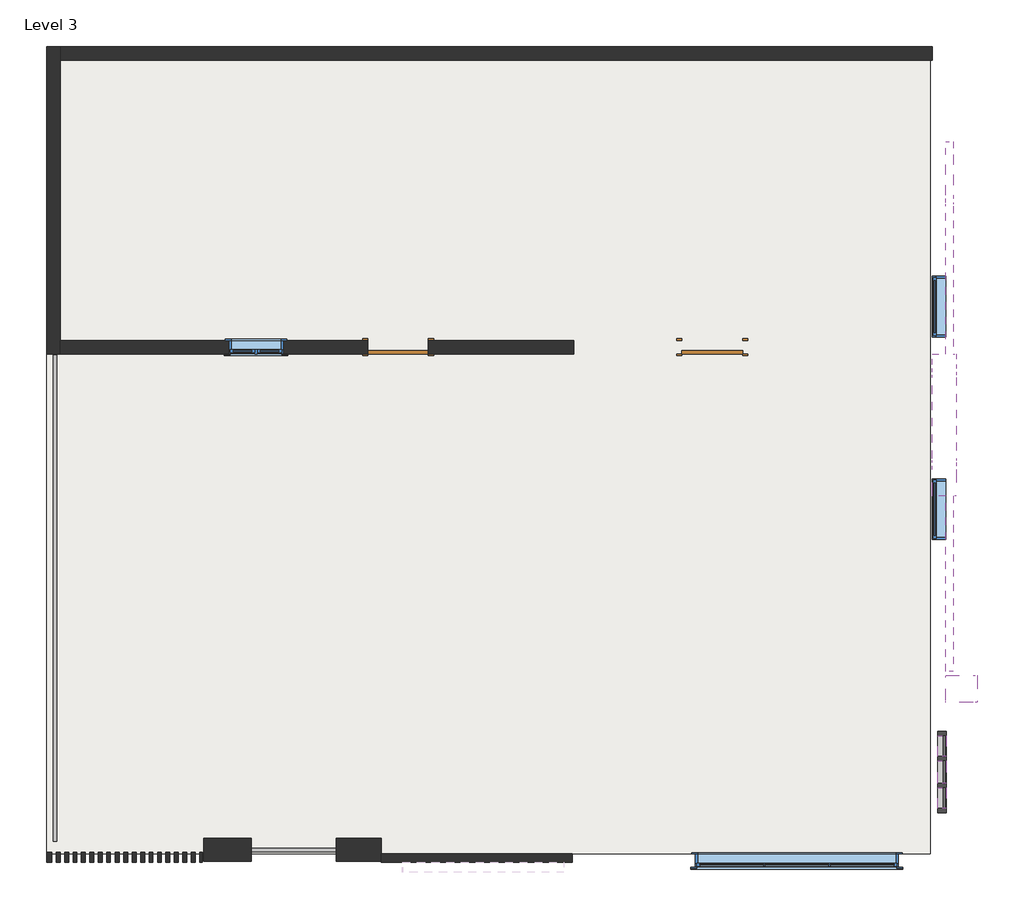
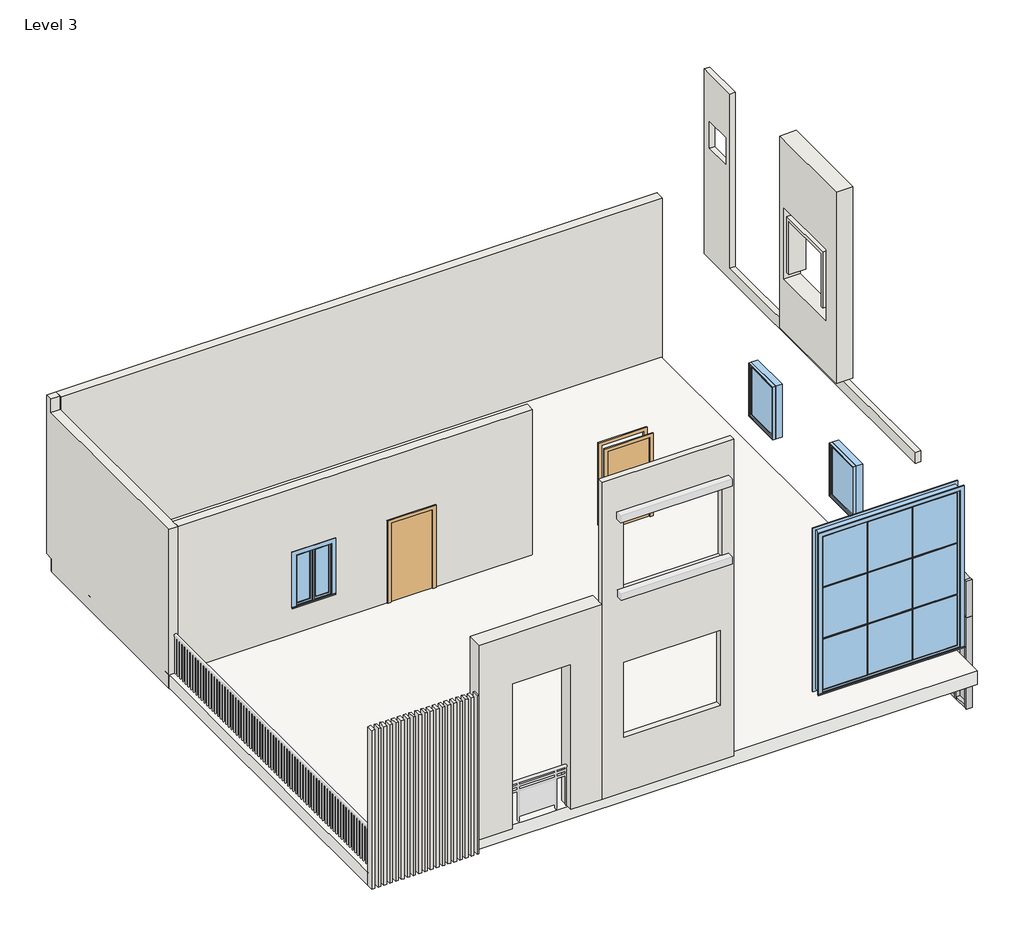
# One storey, part 1 of 2: 24 members, 9 plates, 7 walls, 5 windows, 2 doors, 1 roof.
"""IFC4 building model written with IfcOpenShell, lengths in millimetres."""

from ifc_helpers import new_model, si_unit, frame, origin, place, context, project, spatial, polyline, outline, extrude, faceted_brep, transform, mapped, element, save
from components import door_54dd4da4, member_ff1b7d8f, member_5ad95953, member_62b9d9f2, member_5aeb4b7d, member_9850ab14, member_238a442c, member_fec1d5e2, member_24c95a33, member_92f44db0, member_86adc6a2, system_panel_glazed_2f2cf5d5, system_panel_glazed_6255ac7b, system_panel_glazed_0848ed2a, system_panel_glazed_7089d882, system_panel_glazed_51dabc0a, system_panel_glazed_dcf6fd09, walls_4_walls_4_cd32183e, walls_6_walls_6_5288b44a, window_cae7f124, window_bb17773d, window_8bd8a12f, window_e2841890

model = new_model("IFC4")

# Units and contexts
model_context = context("Model", 3, world=origin())
ifc_project = project(units=[si_unit("LENGTHUNIT", "METRE", prefix="MILLI")], contexts=[model_context])

# Site, building, storey
site = spatial("IfcSite", under=ifc_project)
building = spatial("IfcBuilding", under=site)
storey = spatial("IfcBuildingStorey", under=building, Name="Level 3", Elevation=7315.2)

# Doors
placement = place(None, origin())
door_shape = door_54dd4da4(model_context)
element("IfcDoor", 1, ObjectType="Single-Flush : 36\" x 84\"", at=placement, inside=storey, context=model_context, shape_type="MappedRepresentation", body=[
    mapped(door_shape, transform((-6567.2745124, 6836.8609482, 7315.2), x_axis=(-1.0, 0.0, 0.0), y_axis=(0.0, -1.0, 0.0), z_axis=(0.0, 0.0, 1.0))),
])
element("IfcDoor", 2, ObjectType="Single-Flush : 36\" x 84\"", at=placement, inside=storey, context=model_context, shape_type="MappedRepresentation", body=[
    mapped(door_shape, transform((-1842.8745124, 6836.8609482, 7315.2), x_axis=(-1.0, 0.0, 0.0), y_axis=(0.0, -1.0, 0.0), z_axis=(0.0, 0.0, 1.0))),
])

# Members
member_shape = member_ff1b7d8f(model_context)
element("IfcMember", 3, ObjectType="Rectangular Mullion : 2.5\" x 5\" rectangular", at=placement, inside=storey, context=model_context, shape_type="MappedRepresentation", body=[
    mapped(member_shape, transform((1611.5254876, 617.0832725, 6324.9019988), x_axis=(0.0, 0.0, -1.0), y_axis=(-1.0, 0.0, 0.0), z_axis=(0.0, 1.0, 0.0))),
])
member_2_shape = member_5ad95953(model_context)
element("IfcMember", 4, ObjectType="Rectangular Mullion : 2.5\" x 5\" rectangular", at=placement, inside=storey, context=model_context, shape_type="MappedRepresentation", body=[
    mapped(member_2_shape, transform((1611.5254876, 210.6832725, 6324.9019988), x_axis=(0.0, 0.0, -1.0), y_axis=(-1.0, 0.0, 0.0), z_axis=(0.0, 1.0, 0.0))),
])
element("IfcMember", 5, ObjectType="Rectangular Mullion : 2.5\" x 5\" rectangular", at=placement, inside=storey, context=model_context, shape_type="MappedRepresentation", body=[
    mapped(member_2_shape, transform((1611.5254876, 991.7332725, 6324.9019988), x_axis=(0.0, 0.0, -1.0), y_axis=(-1.0, 0.0, 0.0), z_axis=(0.0, 1.0, 0.0))),
])
member_3_shape = member_62b9d9f2(model_context)
element("IfcMember", 6, ObjectType="Rectangular Mullion : 2.5\" x 5\" rectangular", at=placement, inside=storey, context=model_context, shape_type="MappedRepresentation", body=[
    mapped(member_3_shape, transform((1611.5254876, 242.4332725, 6324.9019988), x_axis=(0.0, -1.0, 0.0), y_axis=(-1.0, 0.0, 0.0), z_axis=(0.0, 0.0, -1.0))),
])
element("IfcMember", 7, ObjectType="Rectangular Mullion : 2.5\" x 5\" rectangular", at=placement, inside=storey, context=model_context, shape_type="MappedRepresentation", body=[
    mapped(member_3_shape, transform((1611.5254876, 648.8332725, 6324.9019988), x_axis=(0.0, -1.0, 0.0), y_axis=(-1.0, 0.0, 0.0), z_axis=(0.0, 0.0, -1.0))),
])
member_4_shape = member_5aeb4b7d(model_context)
element("IfcMember", 8, ObjectType="Rectangular Mullion : 2.5\" x 5\" rectangular", at=placement, inside=storey, context=model_context, shape_type="MappedRepresentation", body=[
    mapped(member_4_shape, transform((1611.5254876, 274.1832725, 7239.0), x_axis=(0.0, 0.0, 1.0), y_axis=(-1.0, 0.0, 0.0), z_axis=(0.0, -1.0, 0.0))),
])
element("IfcMember", 9, ObjectType="Rectangular Mullion : 2.5\" x 5\" rectangular", at=placement, inside=storey, context=model_context, shape_type="MappedRepresentation", body=[
    mapped(member_4_shape, transform((1611.5254876, 274.1832725, 8433.1019988), x_axis=(0.0, 0.0, 1.0), y_axis=(-1.0, 0.0, 0.0), z_axis=(0.0, -1.0, 0.0))),
])
member_5_shape = member_9850ab14(model_context)
element("IfcMember", 10, ObjectType="Rectangular Mullion : 2.5\" x 5\" rectangular", at=placement, inside=storey, context=model_context, shape_type="MappedRepresentation", body=[
    mapped(member_5_shape, transform((1611.5254876, -100.4667275, 7239.0), x_axis=(0.0, 0.0, 1.0), y_axis=(-1.0, 0.0, 0.0), z_axis=(0.0, -1.0, 0.0))),
])
element("IfcMember", 11, ObjectType="Rectangular Mullion : 2.5\" x 5\" rectangular", at=placement, inside=storey, context=model_context, shape_type="MappedRepresentation", body=[
    mapped(member_5_shape, transform((1611.5254876, 680.5832725, 7239.0), x_axis=(0.0, 0.0, 1.0), y_axis=(-1.0, 0.0, 0.0), z_axis=(0.0, -1.0, 0.0))),
])
element("IfcMember", 12, ObjectType="Rectangular Mullion : 2.5\" x 5\" rectangular", at=placement, inside=storey, context=model_context, shape_type="MappedRepresentation", body=[
    mapped(member_5_shape, transform((1611.5254876, -100.4667275, 8433.1019988), x_axis=(0.0, 0.0, 1.0), y_axis=(-1.0, 0.0, 0.0), z_axis=(0.0, -1.0, 0.0))),
])
element("IfcMember", 13, ObjectType="Rectangular Mullion : 2.5\" x 5\" rectangular", at=placement, inside=storey, context=model_context, shape_type="MappedRepresentation", body=[
    mapped(member_5_shape, transform((1611.5254876, 680.5832725, 8433.1019988), x_axis=(0.0, 0.0, 1.0), y_axis=(-1.0, 0.0, 0.0), z_axis=(0.0, -1.0, 0.0))),
])
member_6_shape = member_238a442c(model_context)
element("IfcMember", 14, ObjectType="Rectangular Mullion : 2.5\" x 5\" rectangular", at=placement, inside=storey, context=model_context, shape_type="MappedRepresentation", body=[
    mapped(member_6_shape, transform((1611.5254876, 1055.2332725, 7239.0), x_axis=(0.0, 1.0, 0.0), y_axis=(-1.0, 0.0, 0.0), z_axis=(0.0, 0.0, 1.0))),
])
element("IfcMember", 15, ObjectType="Rectangular Mullion : 2.5\" x 5\" rectangular", at=placement, inside=storey, context=model_context, shape_type="MappedRepresentation", body=[
    mapped(member_6_shape, transform((1611.5254876, -163.9667275, 6324.9019988), x_axis=(0.0, -1.0, 0.0), y_axis=(-1.0, 0.0, 0.0), z_axis=(0.0, 0.0, -1.0))),
])
member_7_shape = member_fec1d5e2(model_context)
element("IfcMember", 16, ObjectType="Rectangular Mullion : 2.5\" x 5\" rectangular", at=placement, inside=storey, context=model_context, shape_type="MappedRepresentation", body=[
    mapped(member_7_shape, transform((1611.5254876, 242.4332725, 7239.0), x_axis=(0.0, -1.0, 0.0), y_axis=(-1.0, 0.0, 0.0), z_axis=(0.0, 0.0, -1.0))),
])
element("IfcMember", 17, ObjectType="Rectangular Mullion : 2.5\" x 5\" rectangular", at=placement, inside=storey, context=model_context, shape_type="MappedRepresentation", body=[
    mapped(member_7_shape, transform((1611.5254876, 648.8332725, 7239.0), x_axis=(0.0, -1.0, 0.0), y_axis=(-1.0, 0.0, 0.0), z_axis=(0.0, 0.0, -1.0))),
])
member_8_shape = member_24c95a33(model_context)
element("IfcMember", 18, ObjectType="Rectangular Mullion : 2.5\" x 5\" rectangular", at=placement, inside=storey, context=model_context, shape_type="MappedRepresentation", body=[
    mapped(member_8_shape, transform((1611.5254876, 1055.2332725, 8433.1019988), x_axis=(0.0, 1.0, 0.0), y_axis=(-1.0, 0.0, 0.0), z_axis=(0.0, 0.0, 1.0))),
])
element("IfcMember", 19, ObjectType="Rectangular Mullion : 2.5\" x 5\" rectangular", at=placement, inside=storey, context=model_context, shape_type="MappedRepresentation", body=[
    mapped(member_8_shape, transform((1611.5254876, -163.9667275, 7239.0), x_axis=(0.0, -1.0, 0.0), y_axis=(-1.0, 0.0, 0.0), z_axis=(0.0, 0.0, -1.0))),
])
member_9_shape = member_92f44db0(model_context)
element("IfcMember", 20, ObjectType="Rectangular Mullion : 2.5\" x 5\" rectangular", at=placement, inside=storey, context=model_context, shape_type="MappedRepresentation", body=[
    mapped(member_9_shape, transform((1611.5254876, 242.4332725, 8433.1019988), x_axis=(0.0, -1.0, 0.0), y_axis=(-1.0, 0.0, 0.0), z_axis=(0.0, 0.0, -1.0))),
])
element("IfcMember", 21, ObjectType="Rectangular Mullion : 2.5\" x 5\" rectangular", at=placement, inside=storey, context=model_context, shape_type="MappedRepresentation", body=[
    mapped(member_9_shape, transform((1611.5254876, 648.8332725, 8433.1019988), x_axis=(0.0, -1.0, 0.0), y_axis=(-1.0, 0.0, 0.0), z_axis=(0.0, 0.0, -1.0))),
])
element("IfcMember", 22, ObjectType="Rectangular Mullion : 2.5\" x 5\" rectangular", at=placement, inside=storey, context=model_context, shape_type="MappedRepresentation", body=[
    mapped(member_2_shape, transform((1611.5254876, 680.5832725, 9271.3019988), x_axis=(0.0, 0.0, 1.0), y_axis=(-1.0, 0.0, 0.0), z_axis=(0.0, -1.0, 0.0))),
])
element("IfcMember", 23, ObjectType="Rectangular Mullion : 2.5\" x 5\" rectangular", at=placement, inside=storey, context=model_context, shape_type="MappedRepresentation", body=[
    mapped(member_2_shape, transform((1611.5254876, -100.4667275, 9271.3019988), x_axis=(0.0, 0.0, 1.0), y_axis=(-1.0, 0.0, 0.0), z_axis=(0.0, -1.0, 0.0))),
])
element("IfcMember", 24, ObjectType="Rectangular Mullion : 2.5\" x 5\" rectangular", at=placement, inside=storey, context=model_context, shape_type="MappedRepresentation", body=[
    mapped(member_shape, transform((1611.5254876, 274.1832725, 9271.3019988), x_axis=(0.0, 0.0, 1.0), y_axis=(-1.0, 0.0, 0.0), z_axis=(0.0, -1.0, 0.0))),
])
member_10_shape = member_86adc6a2(model_context)
element("IfcMember", 25, ObjectType="Rectangular Mullion : 2.5\" x 5\" rectangular", at=placement, inside=storey, context=model_context, shape_type="MappedRepresentation", body=[
    mapped(member_10_shape, transform((1611.5254876, 1055.2332725, 9271.3019988), x_axis=(0.0, 1.0, 0.0), y_axis=(-1.0, 0.0, 0.0), z_axis=(0.0, 0.0, 1.0))),
])
element("IfcMember", 26, ObjectType="Rectangular Mullion : 2.5\" x 5\" rectangular", at=placement, inside=storey, context=model_context, shape_type="MappedRepresentation", body=[
    mapped(member_10_shape, transform((1611.5254876, -163.9667275, 8433.1019988), x_axis=(0.0, -1.0, 0.0), y_axis=(-1.0, 0.0, 0.0), z_axis=(0.0, 0.0, -1.0))),
])

# Plates
system_panel_glazed_shape = system_panel_glazed_2f2cf5d5(model_context)
element("IfcPlate", 27, ObjectType="System Panel : Glazed", at=placement, inside=storey, context=model_context, shape_type="MappedRepresentation", body=[
    mapped(system_panel_glazed_shape, transform((1611.5254876, 836.1582725, 6388.4019988), x_axis=(0.0, -1.0, 0.0), y_axis=(1.0, 0.0, 0.0), z_axis=(0.0, 0.0, 1.0))),
])
element("IfcPlate", 28, ObjectType="System Panel : Glazed", at=placement, inside=storey, context=model_context, shape_type="MappedRepresentation", body=[
    mapped(system_panel_glazed_shape, transform((1611.5254876, 55.1082725, 6388.4019988), x_axis=(0.0, -1.0, 0.0), y_axis=(1.0, 0.0, 0.0), z_axis=(0.0, 0.0, 1.0))),
])
system_panel_glazed_2_shape = system_panel_glazed_6255ac7b(model_context)
element("IfcPlate", 29, ObjectType="System Panel : Glazed", at=placement, inside=storey, context=model_context, shape_type="MappedRepresentation", body=[
    mapped(system_panel_glazed_2_shape, transform((1611.5254876, 445.6332725, 6388.4019988), x_axis=(0.0, -1.0, 0.0), y_axis=(1.0, 0.0, 0.0), z_axis=(0.0, 0.0, 1.0))),
])
system_panel_glazed_3_shape = system_panel_glazed_0848ed2a(model_context)
element("IfcPlate", 30, ObjectType="System Panel : Glazed", at=placement, inside=storey, context=model_context, shape_type="MappedRepresentation", body=[
    mapped(system_panel_glazed_3_shape, transform((1611.5254876, 836.1582725, 7270.75), x_axis=(0.0, -1.0, 0.0), y_axis=(1.0, 0.0, 0.0), z_axis=(0.0, 0.0, 1.0))),
])
element("IfcPlate", 31, ObjectType="System Panel : Glazed", at=placement, inside=storey, context=model_context, shape_type="MappedRepresentation", body=[
    mapped(system_panel_glazed_3_shape, transform((1611.5254876, 55.1082725, 7270.75), x_axis=(0.0, -1.0, 0.0), y_axis=(1.0, 0.0, 0.0), z_axis=(0.0, 0.0, 1.0))),
])
system_panel_glazed_4_shape = system_panel_glazed_7089d882(model_context)
element("IfcPlate", 32, ObjectType="System Panel : Glazed", at=placement, inside=storey, context=model_context, shape_type="MappedRepresentation", body=[
    mapped(system_panel_glazed_4_shape, transform((1611.5254876, 445.6332725, 7270.75), x_axis=(0.0, -1.0, 0.0), y_axis=(1.0, 0.0, 0.0), z_axis=(0.0, 0.0, 1.0))),
])
system_panel_glazed_5_shape = system_panel_glazed_51dabc0a(model_context)
element("IfcPlate", 33, ObjectType="System Panel : Glazed", at=placement, inside=storey, context=model_context, shape_type="MappedRepresentation", body=[
    mapped(system_panel_glazed_5_shape, transform((1611.5254876, 836.1582725, 8464.8519988), x_axis=(0.0, -1.0, 0.0), y_axis=(1.0, 0.0, 0.0), z_axis=(0.0, 0.0, 1.0))),
])
element("IfcPlate", 34, ObjectType="System Panel : Glazed", at=placement, inside=storey, context=model_context, shape_type="MappedRepresentation", body=[
    mapped(system_panel_glazed_5_shape, transform((1611.5254876, 55.1082725, 8464.8519988), x_axis=(0.0, -1.0, 0.0), y_axis=(1.0, 0.0, 0.0), z_axis=(0.0, 0.0, 1.0))),
])
system_panel_glazed_6_shape = system_panel_glazed_dcf6fd09(model_context)
element("IfcPlate", 35, ObjectType="System Panel : Glazed", at=placement, inside=storey, context=model_context, shape_type="MappedRepresentation", body=[
    mapped(system_panel_glazed_6_shape, transform((1611.5254876, 445.6332725, 8464.8519988), x_axis=(0.0, -1.0, 0.0), y_axis=(1.0, 0.0, 0.0), z_axis=(0.0, 0.0, 1.0))),
])

# Roof
element("IfcRoof", 36, ObjectType="Generic - 12\"", at=placement, inside=storey, context=model_context, shape_type="SweptSolid", body=[
    extrude(outline(polyline([(-11847.2995124, 11192.9609482), (1433.7254876, 11192.9609482), (1433.7254876, -783.1390518), (-11847.2995124, -783.1390518), (-11847.2995124, 11192.9609482)])), frame((0.0, 0.0, 7315.2), z_axis=(0.0, 0.0, 1.0), x_axis=(1.0, 0.0, 0.0)), (0.0, 0.0, 1.0), 304.8),
])

# Walls
element("IfcWall", 37, ObjectType="Generic - 5\"", at=placement, inside=storey, context=model_context, shape_type="SweptSolid", body=[
    extrude(outline(polyline([(7623.0321664, -6816.4084212), (7623.0321664, -3950.544029), (14935.2, -3950.544029), (14935.2, -6816.4084212), (7623.0321664, -6816.4084212)]), holes=[polyline([(13989.7022407, -4213.8822527), (12313.3022407, -4213.8822527), (12313.3022407, -6354.4547188), (13989.7022407, -6354.4547188), (13989.7022407, -4213.8822527)]), polyline([(10627.4720431, -4247.1363239), (8900.2720431, -4247.1363239), (8900.2720431, -6354.4547188), (10627.4720431, -6354.4547188), (10627.4720431, -4247.1363239)])]), frame((0.0, -909.5189974, 0.0), z_axis=(0.0, 1.0, 0.0), x_axis=(0.0, 0.0, 1.0)), (0.0, 0.0, 1.0), 127.0),
])
element("IfcWall", 38, ObjectType="Generic - 6\"", at=placement, inside=storey, context=model_context, shape_type="SweptSolid", body=[
    extrude(outline(polyline([(-11774.3919854, -910.1390518), (-11847.2995124, -910.1390518), (-11847.2995124, -757.7390518), (-11774.3919854, -757.7390518), (-11774.3919854, -910.1390518)])), frame((0.0, 0.0, 7315.2), z_axis=(0.0, 0.0, 1.0), x_axis=(1.0, 0.0, 0.0)), (0.0, 0.0, 1.0), 3657.6),
    extrude(outline(polyline([(-9510.4995124, -910.1390518), (-9547.5440884, -910.1390518), (-9547.5440884, -757.7390518), (-9510.4995124, -757.7390518), (-9510.4995124, -910.1390518)])), frame((0.0, 0.0, 7315.2), z_axis=(0.0, 0.0, 1.0), x_axis=(1.0, 0.0, 0.0)), (0.0, 0.0, 1.0), 3657.6),
    extrude(outline(polyline([(-11647.2745124, -910.1390518), (-11706.5440884, -910.1390518), (-11706.5440884, -757.7390518), (-11647.2745124, -757.7390518), (-11647.2745124, -910.1390518)])), frame((0.0, 0.0, 7315.2), z_axis=(0.0, 0.0, 1.0), x_axis=(1.0, 0.0, 0.0)), (0.0, 0.0, 1.0), 3657.6),
    extrude(outline(polyline([(-11520.3919854, -910.1390518), (-11579.4266155, -910.1390518), (-11579.4266155, -757.7390518), (-11520.3919854, -757.7390518), (-11520.3919854, -910.1390518)])), frame((0.0, 0.0, 7315.2), z_axis=(0.0, 0.0, 1.0), x_axis=(1.0, 0.0, 0.0)), (0.0, 0.0, 1.0), 3657.6),
    extrude(outline(polyline([(-11393.3919854, -910.1390518), (-11452.5440884, -910.1390518), (-11452.5440884, -757.7390518), (-11393.3919854, -757.7390518), (-11393.3919854, -910.1390518)])), frame((0.0, 0.0, 7315.2), z_axis=(0.0, 0.0, 1.0), x_axis=(1.0, 0.0, 0.0)), (0.0, 0.0, 1.0), 3657.6),
    extrude(outline(polyline([(-11266.3919854, -910.1390518), (-11325.5440884, -910.1390518), (-11325.5440884, -757.7390518), (-11266.3919854, -757.7390518), (-11266.3919854, -910.1390518)])), frame((0.0, 0.0, 7315.2), z_axis=(0.0, 0.0, 1.0), x_axis=(1.0, 0.0, 0.0)), (0.0, 0.0, 1.0), 3657.6),
    extrude(outline(polyline([(-11139.3919854, -910.1390518), (-11198.5440884, -910.1390518), (-11198.5440884, -757.7390518), (-11139.3919854, -757.7390518), (-11139.3919854, -910.1390518)])), frame((0.0, 0.0, 7315.2), z_axis=(0.0, 0.0, 1.0), x_axis=(1.0, 0.0, 0.0)), (0.0, 0.0, 1.0), 3657.6),
    extrude(outline(polyline([(-11012.3919854, -910.1390518), (-11071.5440884, -910.1390518), (-11071.5440884, -757.7390518), (-11012.3919854, -757.7390518), (-11012.3919854, -910.1390518)])), frame((0.0, 0.0, 7315.2), z_axis=(0.0, 0.0, 1.0), x_axis=(1.0, 0.0, 0.0)), (0.0, 0.0, 1.0), 3657.6),
    extrude(outline(polyline([(-10893.7440884, -910.1390518), (-10944.5440884, -910.1390518), (-10944.5440884, -757.7390518), (-10893.7440884, -757.7390518), (-10893.7440884, -910.1390518)])), frame((0.0, 0.0, 7315.2), z_axis=(0.0, 0.0, 1.0), x_axis=(1.0, 0.0, 0.0)), (0.0, 0.0, 1.0), 3657.6),
    extrude(outline(polyline([(-10758.3919854, -910.1390518), (-10817.5440884, -910.1390518), (-10817.5440884, -757.7390518), (-10758.3919854, -757.7390518), (-10758.3919854, -910.1390518)])), frame((0.0, 0.0, 7315.2), z_axis=(0.0, 0.0, 1.0), x_axis=(1.0, 0.0, 0.0)), (0.0, 0.0, 1.0), 3657.6),
    extrude(outline(polyline([(-10631.3919854, -910.1390518), (-10690.5440884, -910.1390518), (-10690.5440884, -757.7390518), (-10631.3919854, -757.7390518), (-10631.3919854, -910.1390518)])), frame((0.0, 0.0, 7315.2), z_axis=(0.0, 0.0, 1.0), x_axis=(1.0, 0.0, 0.0)), (0.0, 0.0, 1.0), 3657.6),
    extrude(outline(polyline([(-10504.3919854, -910.1390518), (-10563.5440884, -910.1390518), (-10563.5440884, -757.7390518), (-10504.3919854, -757.7390518), (-10504.3919854, -910.1390518)])), frame((0.0, 0.0, 7315.2), z_axis=(0.0, 0.0, 1.0), x_axis=(1.0, 0.0, 0.0)), (0.0, 0.0, 1.0), 3657.6),
    extrude(outline(polyline([(-10377.3919854, -910.1390518), (-10436.5440884, -910.1390518), (-10436.5440884, -757.7390518), (-10377.3919854, -757.7390518), (-10377.3919854, -910.1390518)])), frame((0.0, 0.0, 7315.2), z_axis=(0.0, 0.0, 1.0), x_axis=(1.0, 0.0, 0.0)), (0.0, 0.0, 1.0), 3657.6),
    extrude(outline(polyline([(-10250.3919854, -910.1390518), (-10309.5440884, -910.1390518), (-10309.5440884, -757.7390518), (-10250.3919854, -757.7390518), (-10250.3919854, -910.1390518)])), frame((0.0, 0.0, 7315.2), z_axis=(0.0, 0.0, 1.0), x_axis=(1.0, 0.0, 0.0)), (0.0, 0.0, 1.0), 3657.6),
    extrude(outline(polyline([(-10123.3919854, -910.1390518), (-10182.5440884, -910.1390518), (-10182.5440884, -757.7390518), (-10123.3919854, -757.7390518), (-10123.3919854, -910.1390518)])), frame((0.0, 0.0, 7315.2), z_axis=(0.0, 0.0, 1.0), x_axis=(1.0, 0.0, 0.0)), (0.0, 0.0, 1.0), 3657.6),
    extrude(outline(polyline([(-9996.3919854, -910.1390518), (-10055.5440884, -910.1390518), (-10055.5440884, -757.7390518), (-9996.3919854, -757.7390518), (-9996.3919854, -910.1390518)])), frame((0.0, 0.0, 7315.2), z_axis=(0.0, 0.0, 1.0), x_axis=(1.0, 0.0, 0.0)), (0.0, 0.0, 1.0), 3657.6),
    extrude(outline(polyline([(-9869.3919854, -910.1390518), (-9928.5440884, -910.1390518), (-9928.5440884, -757.7390518), (-9869.3919854, -757.7390518), (-9869.3919854, -910.1390518)])), frame((0.0, 0.0, 7315.2), z_axis=(0.0, 0.0, 1.0), x_axis=(1.0, 0.0, 0.0)), (0.0, 0.0, 1.0), 3657.6),
    extrude(outline(polyline([(-9742.3919854, -910.1390518), (-9801.5440884, -910.1390518), (-9801.5440884, -757.7390518), (-9742.3919854, -757.7390518), (-9742.3919854, -910.1390518)])), frame((0.0, 0.0, 7315.2), z_axis=(0.0, 0.0, 1.0), x_axis=(1.0, 0.0, 0.0)), (0.0, 0.0, 1.0), 3657.6),
    extrude(outline(polyline([(-9615.3919854, -910.1390518), (-9674.5440884, -910.1390518), (-9674.5440884, -757.7390518), (-9615.3919854, -757.7390518), (-9615.3919854, -910.1390518)])), frame((0.0, 0.0, 7315.2), z_axis=(0.0, 0.0, 1.0), x_axis=(1.0, 0.0, 0.0)), (0.0, 0.0, 1.0), 3657.6),
])
element("IfcWall", 39, ObjectType="Generic - 8\"", at=placement, inside=storey, context=model_context, shape_type="Brep", body=[
    faceted_brep([(-11647.2745124, 11154.8609482, 11277.6), (-11647.2745124, 11154.8609482, 7315.2), (1459.1254876, 11154.8609482, 7315.2), (1459.1254876, 11154.8609482, 8130.9177257), (1459.1254876, 11154.8609482, 10244.4876686), (1459.1254876, 11154.8609482, 11277.6), (-11647.2745124, 11358.0609482, 7315.2), (-11647.2745124, 11358.0609482, 7620.0), (-11647.2745124, 11358.0609482, 7623.0321664), (-11647.2745124, 11358.0609482, 11277.6), (1459.1254876, 11358.0609482, 11277.6), (1459.1254876, 11358.0609482, 7315.2), (1459.1254876, 11345.3609482, 11277.6), (-11647.2745124, 11192.9609482, 11277.6)], [[[0, 1, 2, 3, 4, 5]], [[6, 7, 8, 9, 10, 11]], [[2, 1, 6, 11]], [[0, 5, 12, 10, 9, 13]], [[0, 13, 9, 8, 7, 6, 1]], [[2, 11, 10, 12, 5, 4, 3]]]),
])
element("IfcWall", 40, ObjectType="Generic - 8\"", at=placement, inside=storey, context=model_context, shape_type="Brep", body=[
    faceted_brep([(-11850.4745124, 11154.8609482, 7623.0321664), (-11850.4745124, 11154.8609482, 7620.0), (-11850.4745124, 11154.8609482, 7315.2), (-11850.4745124, 6735.2609482, 7315.2), (-11850.4745124, 6735.2609482, 10972.8), (-11850.4745124, 6786.0609482, 10972.8), (-11850.4745124, 11192.9609482, 10972.8), (-11850.4745124, 11192.9609482, 11277.6), (-11850.4745124, 11358.0609482, 11277.6), (-11850.4745124, 11358.0609482, 7623.0321664), (-11647.2745124, 11154.8609482, 7315.2), (-11647.2745124, 11154.8609482, 7623.0321664), (-11647.2745124, 11358.0609482, 7623.0321664), (-11647.2745124, 11358.0609482, 11277.6), (-11647.2745124, 11192.9609482, 11277.6), (-11647.2745124, 11192.9609482, 10972.8), (-11647.2745124, 6938.4609482, 10972.8), (-11647.2745124, 6735.2609482, 10972.8), (-11647.2745124, 6735.2609482, 7315.2), (-11647.2745124, 6938.4609482, 7315.2)], [[[0, 1, 2, 3, 4, 5, 6, 7, 8, 9]], [[10, 11, 12, 13, 14, 15, 16, 17, 18, 19]], [[3, 2, 10, 19, 18]], [[3, 18, 17, 4]], [[9, 12, 11, 0]], [[0, 11, 10, 2, 1]], [[9, 8, 13, 12]], [[8, 7, 14, 13]], [[14, 7, 6, 15]], [[6, 5, 4, 17, 16, 15]]]),
])
element("IfcWall", 41, ObjectType="Generic - 8\"", at=placement, inside=storey, context=model_context, shape_type="Brep", body=[
    faceted_brep([(-7024.4745124, 6938.4609482, 9448.8), (-7024.4745124, 6938.4609482, 7315.2), (-11647.2745124, 6938.4609482, 7315.2), (-11647.2745124, 6938.4609482, 10972.8), (-3925.6745124, 6938.4609482, 10972.8), (-3925.6745124, 6938.4609482, 7315.2), (-6110.0745124, 6938.4609482, 7315.2), (-6110.0745124, 6938.4609482, 9448.8), (-9107.2745124, 6938.4609482, 9448.8), (-9107.2745124, 6938.4609482, 8229.6), (-8294.4745124, 6938.4609482, 8229.6), (-8294.4745124, 6938.4609482, 9448.8), (-11647.2745124, 6735.2609482, 7315.2), (-7024.4745124, 6735.2609482, 7315.2), (-7024.4745124, 6735.2609482, 9448.8), (-6110.0745124, 6735.2609482, 9448.8), (-6110.0745124, 6735.2609482, 7315.2), (-3925.6745124, 6735.2609482, 7315.2), (-3925.6745124, 6735.2609482, 10972.8), (-11647.2745124, 6735.2609482, 10972.8), (-11647.2745124, 6735.2609482, 7620.0), (-9107.2745124, 6735.2609482, 9448.8), (-8294.4745124, 6735.2609482, 9448.8), (-8294.4745124, 6735.2609482, 8229.6), (-9107.2745124, 6735.2609482, 8229.6)], [[[0, 1, 2, 3, 4, 5, 6, 7], [8, 9, 10, 11]], [[12, 13, 14, 15, 16, 17, 18, 19, 20], [21, 22, 23, 24]], [[2, 1, 13, 12]], [[6, 5, 17, 16]], [[2, 12, 20, 19, 3]], [[5, 4, 18, 17]], [[4, 3, 19, 18]], [[14, 13, 1, 0]], [[15, 14, 0, 7]], [[16, 15, 7, 6]], [[9, 8, 21, 24]], [[10, 9, 24, 23]], [[11, 10, 23, 22]], [[8, 11, 22, 21]]]),
])
walls_4_walls_4_shape = walls_4_walls_4_cd32183e(model_context)
element("IfcWall", 42, ObjectType="Walls 4 : Walls 4", at=placement, inside=storey, context=model_context, shape_type="MappedRepresentation", body=[
    mapped(walls_4_walls_4_shape, transform((0.0, 0.0, 0.0), x_axis=(1.0, 0.0, 0.0), y_axis=(0.0, 1.0, 0.0), z_axis=(0.0, 0.0, 1.0))),
])
walls_6_walls_6_shape = walls_6_walls_6_5288b44a(model_context)
element("IfcWall", 43, ObjectType="Walls 6 : Walls 6", at=placement, inside=storey, context=model_context, shape_type="MappedRepresentation", body=[
    mapped(walls_6_walls_6_shape, transform((0.0, 0.0, 0.0), x_axis=(1.0, 0.0, 0.0), y_axis=(0.0, 1.0, 0.0), z_axis=(0.0, 0.0, 1.0))),
])

# Windows
window_shape = window_cae7f124(model_context)
element("IfcWindow", 44, ObjectType="Casement 3x3 with Trim : 120\" x 144\"", at=placement, inside=storey, context=model_context, shape_type="MappedRepresentation", body=[
    mapped(window_shape, transform((-572.8745124, -884.7390518, 2963.4316285), x_axis=(-1.0, 0.0, 0.0), y_axis=(0.0, -1.0, 0.0), z_axis=(0.0, 0.0, 1.0))),
])
window_2_shape = window_bb17773d(model_context)
element("IfcWindow", 45, ObjectType="Casement Dbl with Trim : 32\" x 48\"", at=placement, inside=storey, context=model_context, shape_type="MappedRepresentation", body=[
    mapped(window_2_shape, transform((-8700.8745124, 6855.9109482, 7315.2), x_axis=(-1.0, 0.0, 0.0), y_axis=(0.0, -1.0, 0.0), z_axis=(0.0, 0.0, 1.0))),
])
window_3_shape = window_8bd8a12f(model_context)
element("IfcWindow", 46, ObjectType="Fixed : 16\" x 24\"", at=placement, inside=storey, context=model_context, shape_type="MappedRepresentation", body=[
    mapped(window_3_shape, transform((1902.0977685, 1661.2989255, 8222.9562869), x_axis=(0.0, -1.0, 0.0), y_axis=(1.0, 0.0, 0.0), z_axis=(0.0, 0.0, 1.0))),
])
window_4_shape = window_e2841890(model_context)
element("IfcWindow", 47, ObjectType="Fixed : 36\" x 48\"", at=placement, inside=storey, context=model_context, shape_type="MappedRepresentation", body=[
    mapped(window_4_shape, transform((1560.7254876, 4436.5609482, 7315.2), x_axis=(0.0, 1.0, 0.0), y_axis=(-1.0, 0.0, 0.0), z_axis=(0.0, 0.0, 1.0))),
])
element("IfcWindow", 48, ObjectType="Fixed : 36\" x 48\"", at=placement, inside=storey, context=model_context, shape_type="MappedRepresentation", body=[
    mapped(window_4_shape, transform((1560.7254876, 7484.5609482, 7315.2), x_axis=(0.0, 1.0, 0.0), y_axis=(-1.0, 0.0, 0.0), z_axis=(0.0, 0.0, 1.0))),
])

save(model, "model.ifc")

# Revit data of these elements
# Type "Single-Flush : 36\" x 84\""
#   Type Mark = "1"
#   Construction Type Id = "MDOOR"
#   Assembly Code = "C1020"
#   Analytic Construction = "Metal"
#   Thickness = 0' - 2"
#   Heat Transfer Coefficient (U) = 0.651978 BTU/(h·ft²·°F)
#   Height = 7' - 0"
#   Trim Projection Ext = 0' - 1"
#   Trim Projection Int = 0' - 1"
#   Trim Width = 0' - 3"
#   Width = 3' - 0"
#   Define Thermal Properties by = 1
#   Door Material = Door - Panel
#   Frame Material = Door - Frame
#   Visual Light Transmittance = 0
#   Solar Heat Gain Coefficient = 0
#   Function = (empty or 0)
#   Wall Closure = (empty or 0)
# Type "Rectangular Mullion : 2.5\" x 5\" rectangular"
#   built-in parameter 1007304 = 0.416667 (stored number, unit not read)
#   built-in parameter 1007301 = 0.104167 (stored number, unit not read)
#   built-in parameter 1007300 = 0.104167 (stored number, unit not read)
# Type "System Panel : Glazed"
#   Construction Type Id = "GSP4R"
#   Analytic Construction = "1/8 in Pilkington single glazing"
#   Visual Light Transmittance = 0.9
#   Solar Heat Gain Coefficient = 0.86
#   Heat Transfer Coefficient (U) = 1.18115 BTU/(h·ft²·°F)
# Type "Generic - 12\""
#   Assembly Code = "B1020"
#   Layers, outside or top first: 1' - 0" no material (function 1)
# Type "Generic - 5\""
#   Assembly Code = "B2010"
#   Layers, outside or top first: 0' - 5" no material (function 1)
# Type "Generic - 6\""
#   Assembly Code = "B2010"
#   Layers, outside or top first: 0' - 6" no material (function 1)
# Type "Generic - 8\""
#   Assembly Code = "B2010"
#   Layers, outside or top first: 0' - 8" no material (function 1)
# Type "Casement 3x3 with Trim : 120\" x 144\""
#   Type Mark = "10"
#   Construction Type Id = "GSP4R"
#   Assembly Code = "B2020100"
#   Analytic Construction = "1/8 in Pilkington single glazing"
#   Visual Light Transmittance = 0.9
#   Solar Heat Gain Coefficient = 0.78
#   Heat Transfer Coefficient (U) = 0.6496 BTU/(h·ft²·°F)
#   Height = 12' - 0"
#   Default Sill Height = 18' - 0"
#   Trim Projection - Ext. = 0' - 0 1/2"
#   Trim Projection - Int. = 0' - 0 3/4"
#   Trim Width - Exterior = 0' - 3 1/2"
#   Trim Width - Interior = 0' - 3 1/2"
#   Width = 10' - 0"
#   Window Inset = 0' - 0 3/4"
#   Define Thermal Properties by = 1
#   Glass Pane Material = Glass
#   Sash Material = Sash
#   Trim Exterior Material = Trim
#   Trim Interior Material = Trim
#   Wall Closure = (empty or 0)
# Type "Casement Dbl with Trim : 32\" x 48\""
#   Type Mark = "15"
#   Construction Type Id = "GSP4R"
#   Assembly Code = "B2020100"
#   Analytic Construction = "1/8 in Pilkington single glazing"
#   Visual Light Transmittance = 0.9
#   Solar Heat Gain Coefficient = 0.78
#   Heat Transfer Coefficient (U) = 0.6496 BTU/(h·ft²·°F)
#   Height = 4' - 0"
#   Default Sill Height = 3' - 0"
#   Trim Projection - Ext. = 0' - 0 1/2"
#   Trim Projection - Int. = 0' - 0 3/4"
#   Trim Width - Exterior = 0' - 3 1/2"
#   Trim Width - Interior = 0' - 3 1/2"
#   Width = 2' - 8"
#   Window Inset = 0' - 0 3/4"
#   Define Thermal Properties by = 1
#   Glass Pane Material = Glass
#   Sash Material = Sash
#   Trim Exterior Material = Trim
#   Trim Interior Material = Trim
#   Wall Closure = (empty or 0)
# Type "Fixed : 16\" x 24\""
#   Type Mark = "4"
#   Construction Type Id = "GSP4R"
#   Assembly Code = "B2020100"
#   Analytic Construction = "1/8 in Pilkington single glazing"
#   Visual Light Transmittance = 0.9
#   Solar Heat Gain Coefficient = 0.78
#   Heat Transfer Coefficient (U) = 0.6496 BTU/(h·ft²·°F)
#   Height = 2' - 0"
#   Default Sill Height = 3' - 0"
#   Width = 1' - 4"
#   Window Inset = 0' - 0 3/4"
#   Define Thermal Properties by = 1
#   Glass Pane Material = Glass
#   Sash Material = Sash
#   Wall Closure = (empty or 0)
# Type "Fixed : 36\" x 48\""
#   Type Mark = "1"
#   Construction Type Id = "GSP4R"
#   Assembly Code = "B2020100"
#   Analytic Construction = "1/8 in Pilkington single glazing"
#   Visual Light Transmittance = 0.9
#   Solar Heat Gain Coefficient = 0.78
#   Heat Transfer Coefficient (U) = 0.6496 BTU/(h·ft²·°F)
#   Height = 4' - 0"
#   Default Sill Height = 3' - 0"
#   Width = 3' - 0"
#   Window Inset = 0' - 0 3/4"
#   Define Thermal Properties by = 1
#   Glass Pane Material = Glass
#   Sash Material = Sash
#   Wall Closure = (empty or 0)
# Elements 1, 2 (IfcDoor, "Single-Flush : 36\" x 84\"")
#   Phase Created = New Construction
#   Materials on its faces: "Door - Frame", "Door - Panel"
# Elements 3, 4, 5, 6, 7, 8, 9, 10, 11, 12, 13, 14, 15, 16, 17, 18, 19, 20, 21, 22, 23, 24, 25, 26 (IfcMember, "Rectangular Mullion : 2.5\" x 5\" rectangular")
#   Phase Created = New Construction
#   Materials on its faces: "Aluminum"
# Elements 27, 28, 29, 30, 31, 32, 33, 34, 35 (IfcPlate, "System Panel : Glazed")
#   Phase Created = New Construction
#   Materials on its faces: "Glass"
# Element 36 (IfcRoof, "Generic - 12\"")
#   built-in parameter 1001705 = 25 (stored number, unit not read)
#   built-in parameter 1001710 = 33615
#   Phase Created = New Construction
#   Materials on its faces: "Default Roof"
# Element 37 (IfcWall, "Generic - 5\"")
#   built-in parameter 1001111 = 1' - 0.11938"
#   Top Offset = 13' - 0"
#   Base Offset = 1' - 0.11938"
#   wall height = 23' - 11.88062"
#   Phase Created = New Construction
#   Base Constraint = Level 3
#   Top Constraint = Level 4
#   Materials on its faces: "Default Wall"
# Element 38 (IfcWall, "Generic - 6\"")
#   Top Offset = 0' - 0"
#   Base Offset = 0' - 0"
#   Unconnected Height = 12' - 0"
#   wall height = 12' - 0"
#   Phase Created = New Construction
#   Base Constraint = Level 3
#   Materials on its faces: "Default Wall"
# Elements 39, 40 (IfcWall, "Generic - 8\"")
#   Top Offset = 0' - 0"
#   Base Offset = 0' - 0"
#   Unconnected Height = 13' - 0"
#   wall height = 13' - 0"
#   Phase Created = New Construction
#   Base Constraint = Level 3
#   Materials on its faces: "Default Wall"
# Element 41 (IfcWall, "Generic - 8\"")
#   Top Offset = 0' - 0"
#   Base Offset = 0' - 0"
#   Unconnected Height = 12' - 0"
#   wall height = 12' - 0"
#   Phase Created = New Construction
#   Base Constraint = Level 3
#   Materials on its faces: "Default Wall"
# Element 42 (IfcWall, "Walls 4 : Walls 4")
#   Phase Created = New Construction
#   Materials on its faces: "Default Wall"
# Element 43 (IfcWall, "Walls 6 : Walls 6")
#   Phase Created = New Construction
#   Materials on its faces: "Default Wall"
# Element 44 (IfcWindow, "Casement 3x3 with Trim : 120\" x 144\"")
#   Mark = "1"
#   Phase Created = New Construction
#   Materials on its faces: "Sash", "Glass", "Trim"
# Element 45 (IfcWindow, "Casement Dbl with Trim : 32\" x 48\"")
#   Mark = "17"
#   Phase Created = New Construction
#   Materials on its faces: "Sash", "Trim", "Glass"
# Element 46 (IfcWindow, "Fixed : 16\" x 24\"")
#   Mark = "15"
#   Phase Created = New Construction
#   Materials on its faces: "Sash", "Glass"
# Element 47 (IfcWindow, "Fixed : 36\" x 48\"")
#   Mark = "9"
#   Phase Created = New Construction
#   Materials on its faces: "Sash", "Glass"
# Element 48 (IfcWindow, "Fixed : 36\" x 48\"")
#   Mark = "10"
#   Phase Created = New Construction
#   Materials on its faces: "Sash", "Glass"
# Materials
#   "Door - Panel": class "Wood", colour RGB 210 159 95, transparency 0
#   "Door - Frame": colour RGB 118 70 51, transparency 0
#   "Glass": class "Glass", colour RGB 0 128 192, transparency 0.75, Description = "Soda Lime Glass", Cost = 0
#   "Sash": class "Wood", colour RGB 224 178 126, transparency 0
#   "Trim": class "Wood", colour RGB 224 178 126, transparency 0
#   "Aluminum": class "Metal", colour RGB 247 247 247, transparency 0, Description = "Aluminum 6061", Cost = 0
#   "Default Roof": colour RGB 88 101 114, transparency 0
#   "Default Wall": colour RGB 128 128 128, transparency 0
